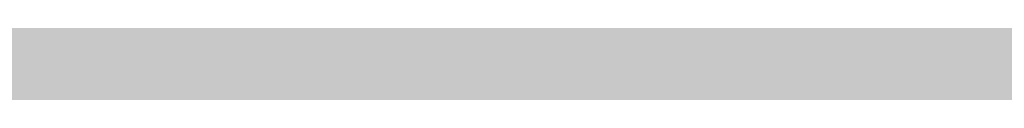
# Model space of a CAD drawing. Units: millimetres. Extents: x 0 to 2267, y 0 to 1823.
# Tile 173 of 256: x 1833.606 to 1838.83, y 1127.583 to 1127.888. Entities that reach past the tile are written whole.
import ezdxf

# ---------------------------------------------------------------- set-up
doc = ezdxf.new("R2010")
doc.units = ezdxf.units.MM
doc.header["$MEASUREMENT"] = 0
doc.layers.add('M-HATC', color=252, linetype='Continuous', lineweight=18)

msp = doc.modelspace()

# ---------------------------------------------------------------- hatches: boundary and pattern name
at = {"layer": 'M-HATC'}
h = msp.add_hatch(color=256, dxfattribs=at)
h.dxf.hatch_style = 1
h.paths.add_polyline_path([(2055.771, 1603.062), (1381.0868, 1603.062), (1381.0868, 1598.062), (2055.771, 1598.062)])
h.paths.add_polyline_path([(2055.771, 1598.062), (1381.0868, 1598.062), (1381.0868, 1593.062), (2055.771, 1593.062)])
h.paths.add_polyline_path([(2051.3074, 1536.7609), (1385.5504, 1536.7609), (1385.5504, 1526.7609), (1387.5504, 1526.7609), (1388.5366, 1525.0528), (1385.3319, 1521.2335), (1385.3319, 1521.2226), (2050.2542, 1522.7491), (2048.3212, 1525.0528), (2049.3074, 1526.7609), (2051.3074, 1526.7609)])
edge = h.paths.add_edge_path()
edge.add_arc((1847.5345, 1379.1492), 135, 222.603061, 222.890851, ccw=False)
edge.add_line((1748.1663, 1287.7656), (1683.0921, 1287.7656))
edge.add_arc((1583.7239, 1379.1492), 135, 317.109149, 317.396939, ccw=False)
edge.add_arc((1678.9686, 1290.6707), 5, 222.8909, 317.1091, ccw=False)
edge.add_arc((1774.2133, 1379.1492), 135, 222.603061, 222.890851, ccw=False)
edge.add_line((1674.8451, 1287.7656), (1609.7709, 1287.7656))
edge.add_arc((1510.4027, 1379.1492), 135, 317.109149, 317.396939, ccw=False)
edge.add_arc((1605.6474, 1290.6707), 5, 222.8909, 317.1091, ccw=False)
edge.add_arc((1700.8921, 1379.1492), 135, 222.603061, 222.890851, ccw=False)
edge.add_line((1601.5239, 1287.7656), (1536.4497, 1287.7656))
edge.add_arc((1437.0815, 1379.1492), 135, 317.109149, 317.396939, ccw=False)
edge.add_arc((1532.3262, 1290.6707), 5, 222.8909, 317.1091, ccw=False)
edge.add_arc((1627.5709, 1379.1492), 135, 222.603061, 222.890851, ccw=False)
edge.add_line((1528.2027, 1287.7656), (1505.9289, 1287.7656))
edge.add_spline(control_points=[(1505.9289, 1287.7656), (1504.2622, 1287.7656), (1504.2622, 1282.7656), (1505.9289, 1282.7656)], knot_values=[0, 0, 0, 0, 5, 5, 5, 5], degree=3, periodic=0)
edge.add_line((1505.9289, 1282.7656), (1930.9289, 1282.7656))
edge.add_spline(control_points=[(1930.9289, 1282.7656), (1932.5956, 1282.7656), (1932.5956, 1287.7656), (1930.9289, 1287.7656)], knot_values=[0, 0, 0, 0, 5, 5, 5, 5], degree=3, periodic=0)
edge.add_line((1930.9289, 1287.7656), (1903.0557, 1287.7656))
edge.add_arc((1803.6875, 1379.1492), 135, 317.109149, 317.396939, ccw=False)
edge.add_arc((1898.9322, 1290.6707), 5, 222.8909, 317.1091, ccw=False)
edge.add_arc((1994.1769, 1379.1492), 135, 222.603061, 222.890851, ccw=False)
edge.add_line((1894.8087, 1287.7656), (1829.7345, 1287.7656))
edge.add_arc((1730.3663, 1379.1492), 135, 317.109149, 317.396939, ccw=False)
edge.add_arc((1825.611, 1290.6707), 5, 222.8909, 317.1091, ccw=False)
edge.add_arc((1920.8557, 1379.1492), 135, 222.603061, 222.890851, ccw=False)
edge.add_line((1821.4875, 1287.7656), (1756.4133, 1287.7656))
edge.add_arc((1657.0451, 1379.1492), 135, 317.109149, 317.396939, ccw=False)
edge.add_arc((1752.2898, 1290.6707), 5, 222.8909, 317.1091, ccw=False)
edge = h.paths.add_edge_path()
edge.add_spline(control_points=[(1843.4289, 1227.2475), (1845.0956, 1227.2475), (1845.0956, 1232.2475), (1843.4289, 1232.2475)], knot_values=[0, 0, 0, 0, 5, 5, 5, 5], degree=3, periodic=0)
edge.add_line((1843.4289, 1232.2475), (1593.4289, 1232.2475))
edge.add_spline(control_points=[(1593.4289, 1232.2475), (1591.7622, 1232.2475), (1591.7622, 1227.2475), (1593.4289, 1227.2475)], knot_values=[0, 0, 0, 0, 5, 5, 5, 5], degree=3, periodic=0)
edge.add_line((1593.4289, 1227.2475), (1843.4289, 1227.2475))
h.paths.add_polyline_path([(1905.9289, 1127.4171), (1530.9289, 1127.4171, 0.414214), (1520.9289, 1117.4171), (1530.9289, 1117.4171), (1915.9289, 1117.4171, 0.414214)])
edge = h.paths.add_edge_path()
edge.add_arc((1397.0858, 1498.4078), 12.7299, 90.78215, 190.87871, ccw=False)
edge.add_line((1396.912, 1511.1365), (1428.0097, 1511.3488))
edge.add_line((1428.0097, 1511.3488), (1433.0097, 1511.3488))
edge.add_line((1433.0097, 1511.3488), (1434.439, 1511.3488))
edge.add_arc((1419.474, 1498.0804), 20, 41.561, 74.08211)
edge.add_line((1424.9592, 1517.3135), (1399.9351, 1517.2561))
edge.add_spline(control_points=[(1399.9307, 1517.2561), (1399.884, 1517.2131), (1399.8328, 1517.1689), (1399.7774, 1517.1236)], knot_values=[11.567499, 11.567499, 11.567499, 11.567499, 11.814249, 11.814249, 11.814249, 11.814249], degree=3, periodic=0)
edge.add_spline(control_points=[(1399.6328, 1517.0099), (1399.5831, 1516.9721), (1399.5307, 1516.9338), (1399.4759, 1516.8947)], knot_values=[11.167718, 11.167718, 11.167718, 11.167718, 11.365188, 11.365188, 11.365188, 11.365188], degree=3, periodic=0)
edge.add_spline(control_points=[(1399.3398, 1516.8001), (1399.1514, 1516.6719), (1398.9384, 1516.5377), (1398.704, 1516.3994)], knot_values=[10.376405, 10.376405, 10.376405, 10.376405, 11.00994, 11.00994, 11.00994, 11.00994], degree=3, periodic=0)
edge.add_spline(control_points=[(1398.6572, 1516.3719), (1398.5789, 1516.326), (1398.4983, 1516.2797), (1398.4155, 1516.2331)], knot_values=[10.125175, 10.125175, 10.125175, 10.125175, 10.334406, 10.334406, 10.334406, 10.334406], degree=3, periodic=0)
edge.add_spline(control_points=[(1398.2642, 1516.1487), (1398.196, 1516.1111), (1398.1263, 1516.0732), (1398.0555, 1516.0351)], knot_values=[9.832246, 9.832246, 9.832246, 9.832246, 9.999658, 9.999658, 9.999658, 9.999658], degree=3, periodic=0)
edge.add_spline(control_points=[(1397.9987, 1516.0048), (1397.7312, 1515.8621), (1397.446, 1515.7171), (1397.1466, 1515.5714)], knot_values=[9.161808, 9.161808, 9.161808, 9.161808, 9.787769, 9.787769, 9.787769, 9.787769], degree=3, periodic=0)
edge.add_spline(control_points=[(1397.1466, 1515.5714), (1396.8418, 1515.423), (1396.5222, 1515.274), (1396.1914, 1515.1262)], knot_values=[8.524455, 8.524455, 8.524455, 8.524455, 9.161808, 9.161808, 9.161808, 9.161808], degree=3, periodic=0)
edge.add_spline(control_points=[(1396.0777, 1515.0756), (1395.9854, 1515.0348), (1395.8922, 1514.994), (1395.7983, 1514.9534)], knot_values=[8.275193, 8.275193, 8.275193, 8.275193, 8.451726, 8.451726, 8.451726, 8.451726], degree=3, periodic=0)
edge.add_spline(control_points=[(1395.6018, 1514.8691), (1395.4997, 1514.8257), (1395.3968, 1514.7824), (1395.2932, 1514.7394)], knot_values=[7.962917, 7.962917, 7.962917, 7.962917, 8.152764, 8.152764, 8.152764, 8.152764], degree=3, periodic=0)
edge.add_spline(control_points=[(1395.2116, 1514.7057), (1394.8278, 1514.5475), (1394.4345, 1514.3929), (1394.0364, 1514.2442)], knot_values=[7.21254, 7.21254, 7.21254, 7.21254, 7.913148, 7.913148, 7.913148, 7.913148], degree=3, periodic=0)
edge.add_spline(control_points=[(1394.0364, 1514.2442), (1393.7076, 1514.1214), (1393.3754, 1514.0027), (1393.0427, 1513.8895)], knot_values=[6.633733, 6.633733, 6.633733, 6.633733, 7.21254, 7.21254, 7.21254, 7.21254], degree=3, periodic=0)
edge.add_spline(control_points=[(1392.8214, 1513.815), (1392.7198, 1513.7812), (1392.6181, 1513.7479), (1392.5166, 1513.7152)], knot_values=[6.328796, 6.328796, 6.328796, 6.328796, 6.505493, 6.505493, 6.505493, 6.505493], degree=3, periodic=0)
edge.add_spline(control_points=[(1392.5166, 1513.7152), (1392.3187, 1513.6515), (1392.1212, 1513.59), (1391.9244, 1513.531)], knot_values=[5.984605, 5.984605, 5.984605, 5.984605, 6.328796, 6.328796, 6.328796, 6.328796], degree=3, periodic=0)
edge.add_spline(control_points=[(1391.7915, 1513.4915), (1391.3122, 1513.3501), (1390.8384, 1513.2239), (1390.3784, 1513.1171)], knot_values=[5.066697, 5.066697, 5.066697, 5.066697, 5.907055, 5.907055, 5.907055, 5.907055], degree=3, periodic=0)
edge.add_spline(control_points=[(1390.3784, 1513.1171), (1390.1797, 1513.071), (1389.9836, 1513.0284), (1389.7907, 1512.9899)], knot_values=[4.70367, 4.70367, 4.70367, 4.70367, 5.066695, 5.066695, 5.066695, 5.066695], degree=3, periodic=0)
edge.add_spline(control_points=[(1389.422, 1512.9204), (1389.2459, 1512.8892), (1389.0729, 1512.8617), (1388.9036, 1512.8381)], knot_values=[4.130571, 4.130571, 4.130571, 4.130571, 4.469816, 4.469816, 4.469816, 4.469816], degree=3, periodic=0)
edge.add_spline(control_points=[(1388.9036, 1512.8381), (1388.591, 1512.7946), (1388.2911, 1512.7644), (1388.0071, 1512.7494)], knot_values=[3.504031, 3.504031, 3.504031, 3.504031, 4.130571, 4.130571, 4.130571, 4.130571], degree=3, periodic=0)
edge.add_spline(control_points=[(1387.9356, 1512.7459), (1387.8538, 1512.7423), (1387.7733, 1512.74), (1387.6944, 1512.739)], knot_values=[3.268866, 3.268866, 3.268866, 3.268866, 3.451164, 3.451164, 3.451164, 3.451164], degree=3, periodic=0)
edge.add_spline(control_points=[(1387.3351, 1512.7443), (1387.2076, 1512.7499), (1387.0847, 1512.7597), (1386.967, 1512.7739)], knot_values=[2.670686, 2.670686, 2.670686, 2.670686, 2.984, 2.984, 2.984, 2.984], degree=3, periodic=0)
edge.add_spline(control_points=[(1386.8327, 1512.7922), (1386.8209, 1512.7941), (1386.8092, 1512.7959), (1386.7975, 1512.7979)], knot_values=[2.516981, 2.516981, 2.516981, 2.516981, 2.549528, 2.549528, 2.549528, 2.549528], degree=3, periodic=0)
edge.add_spline(control_points=[(1386.4526, 1512.8735), (1386.4257, 1512.881), (1386.3993, 1512.889), (1386.3733, 1512.8972)], knot_values=[2.095869, 2.095869, 2.095869, 2.095869, 2.17941, 2.17941, 2.17941, 2.17941], degree=3, periodic=0)
edge.add_spline(control_points=[(1386.0691, 1513.0189), (1386.0634, 1513.0217), (1386.0577, 1513.0246), (1386.052, 1513.0275)], knot_values=[1.72453, 1.72453, 1.72453, 1.72453, 1.745933, 1.745933, 1.745933, 1.745933], degree=3, periodic=0)
edge.add_arc((1399.474, 1498.0804), 20, 131.82432, 180)
edge.add_arc((1630.3336, 1505.5484), 250.9708, 181.705176, 236.427975)
edge.add_arc((1605.3399, 1483.3044), 218.7822, 238.660829, 243.34961)
edge.add_arc((1647.0911, 1510.3592), 262.8986, 183.129836, 237.853442, ccw=False)
h.paths.add_polyline_path([(1406.5369, 1391.9644, 0.149382), (1491.5506, 1296.4418, -0.129517)], flags=17)
edge = h.paths.add_edge_path()
edge.add_arc((2037.3838, 1498.0804), 20, 0, 48.26587)
edge.add_spline(control_points=[(2050.6973, 1513.0052), (2050.6512, 1512.9847), (2050.6034, 1512.9655), (2050.5539, 1512.9477)], knot_values=[1.835652, 1.835652, 1.835652, 1.835652, 2.000781, 2.000781, 2.000781, 2.000781], degree=3, periodic=0)
edge.add_spline(control_points=[(2050.4616, 1512.9166), (2050.479, 1512.9221), (2050.4963, 1512.9277), (2050.5133, 1512.9335)], knot_values=[2.045477, 2.045477, 2.045477, 2.045477, 2.101389, 2.101389, 2.101389, 2.101389], degree=3, periodic=0)
edge.add_spline(control_points=[(2050.129, 1512.8342), (2050.1984, 1512.8473), (2050.2657, 1512.8623), (2050.3308, 1512.8792)], knot_values=[2.237629, 2.237629, 2.237629, 2.237629, 2.435841, 2.435841, 2.435841, 2.435841], degree=3, periodic=0)
edge.add_spline(control_points=[(2050.0946, 1512.8278), (2050.1061, 1512.8299), (2050.1176, 1512.832), (2050.129, 1512.8342)], knot_values=[2.435841, 2.435841, 2.435841, 2.435841, 2.468321, 2.468321, 2.468321, 2.468321], degree=3, periodic=0)
edge.add_spline(control_points=[(2049.7843, 1512.7851), (2049.8552, 1512.7922), (2049.9243, 1512.8008), (2049.9917, 1512.8109)], knot_values=[2.563852, 2.563852, 2.563852, 2.563852, 2.748541, 2.748541, 2.748541, 2.748541], degree=3, periodic=0)
edge.add_spline(control_points=[(2049.4052, 1512.7617), (2049.5364, 1512.7653), (2049.6629, 1512.773), (2049.7843, 1512.7851)], knot_values=[2.748541, 2.748541, 2.748541, 2.748541, 3.064882, 3.064882, 3.064882, 3.064882], degree=3, periodic=0)
edge.add_spline(control_points=[(2049.1698, 1512.7597), (2049.2336, 1512.7591), (2049.2965, 1512.7594), (2049.3584, 1512.7606)], knot_values=[3.102309, 3.102309, 3.102309, 3.102309, 3.2503, 3.2503, 3.2503, 3.2503], degree=3, periodic=0)
edge.add_spline(control_points=[(2048.8573, 1512.7691), (2048.9638, 1512.7638), (2049.068, 1512.7606), (2049.1698, 1512.7597)], knot_values=[3.2503, 3.2503, 3.2503, 3.2503, 3.486069, 3.486069, 3.486069, 3.486069], degree=3, periodic=0)
edge.add_spline(control_points=[(2048.6924, 1512.7789), (2048.3729, 1512.8009), (2048.0345, 1512.8411), (2047.6817, 1512.897)], knot_values=[3.606429, 3.606429, 3.606429, 3.606429, 4.2989, 4.2989, 4.2989, 4.2989], degree=3, periodic=0)
edge.add_spline(control_points=[(2047.6817, 1512.897), (2047.5458, 1512.9185), (2047.4077, 1512.9424), (2047.2678, 1512.9685)], knot_values=[4.2989, 4.2989, 4.2989, 4.2989, 4.565769, 4.565769, 4.565769, 4.565769], degree=3, periodic=0)
edge.add_spline(control_points=[(2047.2678, 1512.9685), (2047.1449, 1512.9914), (2047.0207, 1513.016), (2046.8951, 1513.0422)], knot_values=[4.565769, 4.565769, 4.565769, 4.565769, 4.799971, 4.799971, 4.799971, 4.799971], degree=3, periodic=0)
edge.add_spline(control_points=[(2046.8951, 1513.0422), (2046.5286, 1513.1188), (2046.1513, 1513.209), (2045.7676, 1513.3107)], knot_values=[4.799971, 4.799971, 4.799971, 4.799971, 5.483718, 5.483718, 5.483718, 5.483718], degree=3, periodic=0)
edge.add_spline(control_points=[(2045.7676, 1513.3107), (2045.3724, 1513.4154), (2044.9704, 1513.5322), (2044.5662, 1513.6588)], knot_values=[5.483718, 5.483718, 5.483718, 5.483718, 6.187866, 6.187866, 6.187866, 6.187866], degree=3, periodic=0)
edge.add_spline(control_points=[(2044.5662, 1513.6588), (2044.4149, 1513.7061), (2044.2633, 1513.7549), (2044.1116, 1513.8048)], knot_values=[6.187866, 6.187866, 6.187866, 6.187866, 6.451551, 6.451551, 6.451551, 6.451551], degree=3, periodic=0)
edge.add_spline(control_points=[(2044.1116, 1513.8048), (2043.9967, 1513.8427), (2043.8817, 1513.8813), (2043.7668, 1513.9205)], knot_values=[6.451551, 6.451551, 6.451551, 6.451551, 6.651434, 6.651434, 6.651434, 6.651434], degree=3, periodic=0)
edge.add_spline(control_points=[(2043.7668, 1513.9205), (2043.3716, 1514.0554), (2042.9774, 1514.1979), (2042.5886, 1514.3458)], knot_values=[6.651434, 6.651434, 6.651434, 6.651434, 7.338879, 7.338879, 7.338879, 7.338879], degree=3, periodic=0)
edge.add_spline(control_points=[(2042.5886, 1514.3458), (2042.1643, 1514.5071), (2041.7465, 1514.6749), (2041.3409, 1514.846)], knot_values=[7.338879, 7.338879, 7.338879, 7.338879, 8.089209, 8.089209, 8.089209, 8.089209], degree=3, periodic=0)
edge.add_spline(control_points=[(2041.3409, 1514.846), (2041.1028, 1514.9465), (2040.869, 1515.0481), (2040.6405, 1515.1502)], knot_values=[8.089209, 8.089209, 8.089209, 8.089209, 8.529587, 8.529587, 8.529587, 8.529587], degree=3, periodic=0)
edge.add_spline(control_points=[(2040.51, 1515.2089), (2040.0824, 1515.4022), (2039.6747, 1515.5971), (2039.295, 1515.7894)], knot_values=[8.613818, 8.613818, 8.613818, 8.613818, 9.44571, 9.44571, 9.44571, 9.44571], degree=3, periodic=0)
edge.add_spline(control_points=[(2039.295, 1515.7894), (2039.0618, 1515.9075), (2038.8391, 1516.0246), (2038.6288, 1516.1398)], knot_values=[9.44571, 9.44571, 9.44571, 9.44571, 9.956404, 9.956404, 9.956404, 9.956404], degree=3, periodic=0)
edge.add_spline(control_points=[(2038.6288, 1516.1398), (2038.5187, 1516.2001), (2038.4121, 1516.2598), (2038.309, 1516.3189)], knot_values=[9.956404, 9.956404, 9.956404, 9.956404, 10.223542, 10.223542, 10.223542, 10.223542], degree=3, periodic=0)
edge.add_spline(control_points=[(2038.309, 1516.3189), (2038.2138, 1516.3735), (2038.1216, 1516.4276), (2038.0328, 1516.481)], knot_values=[10.223542, 10.223542, 10.223542, 10.223542, 10.47051, 10.47051, 10.47051, 10.47051], degree=3, periodic=0)
edge.add_spline(control_points=[(2038.0328, 1516.481), (2037.7855, 1516.6296), (2037.5639, 1516.773), (2037.3722, 1516.909)], knot_values=[10.47051, 10.47051, 10.47051, 10.47051, 11.15767, 11.15767, 11.15767, 11.15767], degree=3, periodic=0)
edge.add_spline(control_points=[(2037.3722, 1516.909), (2037.2789, 1516.9752), (2037.1927, 1517.0396), (2037.1142, 1517.102)], knot_values=[11.15767, 11.15767, 11.15767, 11.15767, 11.49227, 11.49227, 11.49227, 11.49227], degree=3, periodic=0)
edge.add_spline(control_points=[(2036.8564, 1517.3259), (2036.9148, 1517.2692), (2036.9814, 1517.2103), (2037.0557, 1517.1492)], knot_values=[11.577341, 11.577341, 11.577341, 11.577341, 11.91035, 11.91035, 11.91035, 11.91035], degree=3, periodic=0)
edge.add_spline(control_points=[(2036.8074, 1517.3748), (2036.823, 1517.3587), (2036.8393, 1517.3424), (2036.8564, 1517.3259)], knot_values=[11.91035, 11.91035, 11.91035, 11.91035, 12.007402, 12.007402, 12.007402, 12.007402], degree=3, periodic=0)
edge.add_spline(control_points=[(2036.7017, 1517.494), (2036.7104, 1517.483), (2036.7196, 1517.4719), (2036.7291, 1517.4606)], knot_values=[12.184155, 12.184155, 12.184155, 12.184155, 12.255409, 12.255409, 12.255409, 12.255409], degree=3, periodic=0)
edge.add_spline(control_points=[(2036.6159, 1517.6205), (2036.62, 1517.613), (2036.6243, 1517.6055), (2036.6289, 1517.5979)], knot_values=[12.487913, 12.487913, 12.487913, 12.487913, 12.541035, 12.541035, 12.541035, 12.541035], degree=3, periodic=0)
edge.add_spline(control_points=[(2036.5635, 1517.786), (2036.5637, 1517.7794), (2036.5642, 1517.7726), (2036.565, 1517.7658)], knot_values=[12.911761, 12.911761, 12.911761, 12.911761, 12.968286, 12.968286, 12.968286, 12.968286], degree=3, periodic=0)
edge.add_spline(control_points=[(2036.6166, 1517.9304), (2036.6125, 1517.9259), (2036.6086, 1517.9212), (2036.6049, 1517.9165)], knot_values=[13.382527, 13.382527, 13.382527, 13.382527, 13.433791, 13.433791, 13.433791, 13.433791], degree=3, periodic=0)
edge.add_spline(control_points=[(2036.749, 1518.017), (2036.7361, 1518.0116), (2036.7239, 1518.006), (2036.7124, 1518.0002)], knot_values=[13.726299, 13.726299, 13.726299, 13.726299, 13.809928, 13.809928, 13.809928, 13.809928], degree=3, periodic=0)
edge.add_spline(control_points=[(2036.8604, 1518.0528), (2036.8386, 1518.0474), (2036.8181, 1518.0416), (2036.7988, 1518.0353)], knot_values=[13.910887, 13.910887, 13.910887, 13.910887, 14.02153, 14.02153, 14.02153, 14.02153], degree=3, periodic=0)
edge.add_line((2036.9639, 1518.0804), (2032.3838, 1518.0804))
edge.add_line((2032.3838, 1518.0804), (2027.3838, 1518.0804))
edge.add_line((2027.3838, 1518.0804), (2022.3838, 1518.0804))
edge.add_line((2022.3838, 1518.0804), (2017.3838, 1518.0804))
edge.add_arc((2017.3838, 1498.0804), 20, 90, 138.439)
edge.add_line((2002.4188, 1511.3488), (2003.8481, 1511.3488))
edge.add_line((2003.8481, 1511.3488), (2008.8481, 1511.3488))
edge.add_line((2008.8481, 1511.3488), (2039.772, 1511.1377))
edge.add_arc((2039.772, 1498.4078), 12.7299, -10.87871, 90, ccw=False)
edge.add_arc((1789.7668, 1510.3592), 262.8986, 302.146558, 356.870164, ccw=False)
edge.add_arc((1831.5179, 1483.3044), 218.7822, 296.65039, 301.339171)
edge.add_arc((1806.5242, 1505.5484), 250.9708, 303.572025, 358.294824)
h.paths.add_polyline_path([(2030.321, 1391.9644, -0.129517), (1945.3072, 1296.4418, 0.149382)], flags=17)
edge = h.paths.add_edge_path()
edge.add_spline(control_points=[(2037.2464, 1518.0821), (2037.2898, 1518.081), (2037.3355, 1518.0804), (2037.3838, 1518.0804)], knot_values=[0.000012, 0.000012, 0.000012, 0.000012, 0.144754, 0.144754, 0.144754, 0.144754], degree=3, periodic=0)
edge.add_line((2037.3357, 1518.0804), (2037.0096, 1518.0804))
edge.add_spline(control_points=[(2037.0096, 1518.0804), (2036.9822, 1518.0768), (2036.956, 1518.0727), (2036.9312, 1518.0681)], knot_values=[14.13465, 14.13465, 14.13465, 14.13465, 14.247197, 14.247197, 14.247197, 14.247197], degree=3, periodic=0)
edge.add_spline(control_points=[(2036.9312, 1518.0681), (2036.9276, 1518.0674), (2036.9241, 1518.0667), (2036.9205, 1518.0661)], knot_values=[14.118315, 14.118315, 14.118315, 14.118315, 14.13465, 14.13465, 14.13465, 14.13465], degree=3, periodic=0)
edge.add_spline(control_points=[(2036.9205, 1518.0661), (2036.9118, 1518.0644), (2036.9032, 1518.0626), (2036.8948, 1518.0608)], knot_values=[14.078086, 14.078086, 14.078086, 14.078086, 14.118315, 14.118315, 14.118315, 14.118315], degree=3, periodic=0)
edge.add_spline(control_points=[(2036.8948, 1518.0608), (2036.883, 1518.0583), (2036.8716, 1518.0556), (2036.8604, 1518.0528)], knot_values=[14.02153, 14.02153, 14.02153, 14.02153, 14.078086, 14.078086, 14.078086, 14.078086], degree=3, periodic=0)
edge.add_spline(control_points=[(2036.8604, 1518.0528), (2036.8386, 1518.0474), (2036.8181, 1518.0416), (2036.7988, 1518.0353)], knot_values=[13.910887, 13.910887, 13.910887, 13.910887, 14.02153, 14.02153, 14.02153, 14.02153], degree=3, periodic=0)
edge.add_spline(control_points=[(2036.7988, 1518.0353), (2036.7981, 1518.035), (2036.7974, 1518.0348), (2036.7967, 1518.0346)], knot_values=[13.906906, 13.906906, 13.906906, 13.906906, 13.910887, 13.910887, 13.910887, 13.910887], degree=3, periodic=0)
edge.add_spline(control_points=[(2036.7967, 1518.0346), (2036.7882, 1518.0318), (2036.7799, 1518.0289), (2036.7719, 1518.0259)], knot_values=[13.857826, 13.857826, 13.857826, 13.857826, 13.906906, 13.906906, 13.906906, 13.906906], degree=3, periodic=0)
edge.add_spline(control_points=[(2036.7719, 1518.0259), (2036.764, 1518.023), (2036.7564, 1518.02), (2036.749, 1518.017)], knot_values=[13.809928, 13.809928, 13.809928, 13.809928, 13.857826, 13.857826, 13.857826, 13.857826], degree=3, periodic=0)
edge.add_spline(control_points=[(2036.749, 1518.017), (2036.7361, 1518.0116), (2036.7239, 1518.006), (2036.7124, 1518.0002)], knot_values=[13.726299, 13.726299, 13.726299, 13.726299, 13.809928, 13.809928, 13.809928, 13.809928], degree=3, periodic=0)
edge.add_spline(control_points=[(2036.7124, 1518.0002), (2036.7121, 1518), (2036.7118, 1517.9999), (2036.7115, 1517.9997)], knot_values=[13.723993, 13.723993, 13.723993, 13.723993, 13.726299, 13.726299, 13.726299, 13.726299], degree=3, periodic=0)
edge.add_spline(control_points=[(2036.7115, 1517.9997), (2036.7063, 1517.9971), (2036.7013, 1517.9944), (2036.6965, 1517.9917)], knot_values=[13.686536, 13.686536, 13.686536, 13.686536, 13.723993, 13.723993, 13.723993, 13.723993], degree=3, periodic=0)
edge.add_spline(control_points=[(2036.6965, 1517.9917), (2036.6919, 1517.9891), (2036.6874, 1517.9865), (2036.6831, 1517.9839)], knot_values=[13.651251, 13.651251, 13.651251, 13.651251, 13.686536, 13.686536, 13.686536, 13.686536], degree=3, periodic=0)
edge.add_spline(control_points=[(2036.6831, 1517.9839), (2036.6764, 1517.9798), (2036.67, 1517.9757), (2036.6639, 1517.9714)], knot_values=[13.596804, 13.596804, 13.596804, 13.596804, 13.651251, 13.651251, 13.651251, 13.651251], degree=3, periodic=0)
edge.add_spline(control_points=[(2036.6639, 1517.9714), (2036.6636, 1517.9712), (2036.6633, 1517.9709), (2036.6629, 1517.9707)], knot_values=[13.593956, 13.593956, 13.593956, 13.593956, 13.596804, 13.596804, 13.596804, 13.596804], degree=3, periodic=0)
edge.add_spline(control_points=[(2036.6629, 1517.9707), (2036.6603, 1517.9689), (2036.6577, 1517.967), (2036.6552, 1517.9651)], knot_values=[13.570322, 13.570322, 13.570322, 13.570322, 13.593956, 13.593956, 13.593956, 13.593956], degree=3, periodic=0)
edge.add_spline(control_points=[(2036.6552, 1517.9651), (2036.6525, 1517.9631), (2036.6499, 1517.9611), (2036.6474, 1517.9591)], knot_values=[13.545477, 13.545477, 13.545477, 13.545477, 13.570322, 13.570322, 13.570322, 13.570322], degree=3, periodic=0)
edge.add_spline(control_points=[(2036.6474, 1517.9591), (2036.6472, 1517.9589), (2036.6471, 1517.9588), (2036.6469, 1517.9587)], knot_values=[13.543931, 13.543931, 13.543931, 13.543931, 13.545477, 13.545477, 13.545477, 13.545477], degree=3, periodic=0)
edge.add_spline(control_points=[(2036.6469, 1517.9587), (2036.6412, 1517.9541), (2036.6358, 1517.9494), (2036.6307, 1517.9447)], knot_values=[13.488237, 13.488237, 13.488237, 13.488237, 13.543931, 13.543931, 13.543931, 13.543931], degree=3, periodic=0)
edge.add_spline(control_points=[(2036.6307, 1517.9447), (2036.6282, 1517.9423), (2036.6257, 1517.9399), (2036.6233, 1517.9374)], knot_values=[13.460307, 13.460307, 13.460307, 13.460307, 13.488237, 13.488237, 13.488237, 13.488237], degree=3, periodic=0)
edge.add_spline(control_points=[(2036.6233, 1517.9374), (2036.6215, 1517.9356), (2036.6198, 1517.9338), (2036.6181, 1517.932)], knot_values=[13.439712, 13.439712, 13.439712, 13.439712, 13.460307, 13.460307, 13.460307, 13.460307], degree=3, periodic=0)
edge.add_spline(control_points=[(2036.6181, 1517.932), (2036.6176, 1517.9315), (2036.6171, 1517.9309), (2036.6166, 1517.9304)], knot_values=[13.433791, 13.433791, 13.433791, 13.433791, 13.439712, 13.439712, 13.439712, 13.439712], degree=3, periodic=0)
edge.add_spline(control_points=[(2036.6166, 1517.9304), (2036.6125, 1517.9259), (2036.6086, 1517.9212), (2036.6049, 1517.9165)], knot_values=[13.382527, 13.382527, 13.382527, 13.382527, 13.433791, 13.433791, 13.433791, 13.433791], degree=3, periodic=0)
edge.add_spline(control_points=[(2036.6049, 1517.9165), (2036.6026, 1517.9135), (2036.6004, 1517.9104), (2036.5982, 1517.9074)], knot_values=[13.350017, 13.350017, 13.350017, 13.350017, 13.382527, 13.382527, 13.382527, 13.382527], degree=3, periodic=0)
edge.add_spline(control_points=[(2036.5982, 1517.9074), (2036.5972, 1517.9059), (2036.5962, 1517.9043), (2036.5952, 1517.9028)], knot_values=[13.333922, 13.333922, 13.333922, 13.333922, 13.350017, 13.350017, 13.350017, 13.350017], degree=3, periodic=0)
edge.add_spline(control_points=[(2036.5952, 1517.9028), (2036.5945, 1517.9018), (2036.5939, 1517.9009), (2036.5933, 1517.8999)], knot_values=[13.323828, 13.323828, 13.323828, 13.323828, 13.333922, 13.333922, 13.333922, 13.333922], degree=3, periodic=0)
edge.add_spline(control_points=[(2036.5933, 1517.8999), (2036.5905, 1517.8955), (2036.5879, 1517.8909), (2036.5855, 1517.8864)], knot_values=[13.277545, 13.277545, 13.277545, 13.277545, 13.323828, 13.323828, 13.323828, 13.323828], degree=3, periodic=0)
edge.add_spline(control_points=[(2036.5855, 1517.8864), (2036.5836, 1517.8827), (2036.5817, 1517.8789), (2036.5801, 1517.8751)], knot_values=[13.240119, 13.240119, 13.240119, 13.240119, 13.277545, 13.277545, 13.277545, 13.277545], degree=3, periodic=0)
edge.add_spline(control_points=[(2036.5801, 1517.8751), (2036.5795, 1517.8739), (2036.579, 1517.8727), (2036.5785, 1517.8715)], knot_values=[13.228211, 13.228211, 13.228211, 13.228211, 13.240119, 13.240119, 13.240119, 13.240119], degree=3, periodic=0)
edge.add_spline(control_points=[(2036.5785, 1517.8715), (2036.578, 1517.8702), (2036.5774, 1517.869), (2036.5769, 1517.8677)], knot_values=[13.215717, 13.215717, 13.215717, 13.215717, 13.228211, 13.228211, 13.228211, 13.228211], degree=3, periodic=0)
edge.add_spline(control_points=[(2036.5769, 1517.8677), (2036.5755, 1517.864), (2036.5741, 1517.8603), (2036.5729, 1517.8565)], knot_values=[13.179847, 13.179847, 13.179847, 13.179847, 13.215717, 13.215717, 13.215717, 13.215717], degree=3, periodic=0)
edge.add_spline(control_points=[(2036.5729, 1517.8565), (2036.5713, 1517.8515), (2036.5699, 1517.8464), (2036.5687, 1517.8413)], knot_values=[13.132017, 13.132017, 13.132017, 13.132017, 13.179847, 13.179847, 13.179847, 13.179847], degree=3, periodic=0)
edge.add_spline(control_points=[(2036.5687, 1517.8413), (2036.5684, 1517.8402), (2036.5682, 1517.8392), (2036.568, 1517.8382)], knot_values=[13.122482, 13.122482, 13.122482, 13.122482, 13.132017, 13.132017, 13.132017, 13.132017], degree=3, periodic=0)
edge.add_spline(control_points=[(2036.568, 1517.8382), (2036.5676, 1517.8363), (2036.5672, 1517.8345), (2036.5669, 1517.8327)], knot_values=[13.105592, 13.105592, 13.105592, 13.105592, 13.122482, 13.122482, 13.122482, 13.122482], degree=3, periodic=0)
edge.add_spline(control_points=[(2036.5669, 1517.8327), (2036.5662, 1517.8292), (2036.5657, 1517.8257), (2036.5652, 1517.8222)], knot_values=[13.074063, 13.074063, 13.074063, 13.074063, 13.105592, 13.105592, 13.105592, 13.105592], degree=3, periodic=0)
edge.add_spline(control_points=[(2036.5652, 1517.8222), (2036.5652, 1517.8222), (2036.5652, 1517.8222), (2036.5652, 1517.8222)], knot_values=[13.074043, 13.074043, 13.074043, 13.074043, 13.074063, 13.074063, 13.074063, 13.074063], degree=3, periodic=0)
edge.add_spline(control_points=[(2036.5652, 1517.8222), (2036.5644, 1517.8164), (2036.5639, 1517.8106), (2036.5636, 1517.8046)], knot_values=[13.021884, 13.021884, 13.021884, 13.021884, 13.074043, 13.074043, 13.074043, 13.074043], degree=3, periodic=0)
edge.add_spline(control_points=[(2036.5636, 1517.8046), (2036.5636, 1517.804), (2036.5636, 1517.8034), (2036.5635, 1517.8028)], knot_values=[13.01674, 13.01674, 13.01674, 13.01674, 13.021884, 13.021884, 13.021884, 13.021884], degree=3, periodic=0)
edge.add_spline(control_points=[(2036.5635, 1517.8028), (2036.5634, 1517.8005), (2036.5634, 1517.7982), (2036.5634, 1517.7958)], knot_values=[12.996438, 12.996438, 12.996438, 12.996438, 13.01674, 13.01674, 13.01674, 13.01674], degree=3, periodic=0)
edge.add_spline(control_points=[(2036.5634, 1517.7958), (2036.5633, 1517.7926), (2036.5634, 1517.7893), (2036.5635, 1517.786)], knot_values=[12.968286, 12.968286, 12.968286, 12.968286, 12.996438, 12.996438, 12.996438, 12.996438], degree=3, periodic=0)
edge.add_spline(control_points=[(2036.5635, 1517.786), (2036.5637, 1517.7794), (2036.5642, 1517.7726), (2036.565, 1517.7658)], knot_values=[12.911761, 12.911761, 12.911761, 12.911761, 12.968286, 12.968286, 12.968286, 12.968286], degree=3, periodic=0)
edge.add_spline(control_points=[(2036.565, 1517.7658), (2036.565, 1517.7657), (2036.565, 1517.7656), (2036.565, 1517.7656)], knot_values=[12.911017, 12.911017, 12.911017, 12.911017, 12.911761, 12.911761, 12.911761, 12.911761], degree=3, periodic=0)
edge.add_spline(control_points=[(2036.565, 1517.7656), (2036.5654, 1517.7625), (2036.5658, 1517.7593), (2036.5663, 1517.7562)], knot_values=[12.88528, 12.88528, 12.88528, 12.88528, 12.911017, 12.911017, 12.911017, 12.911017], degree=3, periodic=0)
edge.add_spline(control_points=[(2036.5663, 1517.7562), (2036.5667, 1517.7534), (2036.5672, 1517.7506), (2036.5677, 1517.7478)], knot_values=[12.862519, 12.862519, 12.862519, 12.862519, 12.88528, 12.88528, 12.88528, 12.88528], degree=3, periodic=0)
edge.add_spline(control_points=[(2036.5677, 1517.7478), (2036.5678, 1517.7474), (2036.5679, 1517.7469), (2036.568, 1517.7465)], knot_values=[12.858885, 12.858885, 12.858885, 12.858885, 12.862519, 12.862519, 12.862519, 12.862519], degree=3, periodic=0)
edge.add_spline(control_points=[(2036.568, 1517.7465), (2036.5692, 1517.7399), (2036.5707, 1517.7332), (2036.5724, 1517.7264)], knot_values=[12.8053, 12.8053, 12.8053, 12.8053, 12.858885, 12.858885, 12.858885, 12.858885], degree=3, periodic=0)
edge.add_spline(control_points=[(2036.5724, 1517.7264), (2036.5734, 1517.7226), (2036.5745, 1517.7187), (2036.5756, 1517.7149)], knot_values=[12.775176, 12.775176, 12.775176, 12.775176, 12.8053, 12.8053, 12.8053, 12.8053], degree=3, periodic=0)
edge.add_spline(control_points=[(2036.5756, 1517.7149), (2036.5763, 1517.7125), (2036.577, 1517.7102), (2036.5778, 1517.7078)], knot_values=[12.756759, 12.756759, 12.756759, 12.756759, 12.775176, 12.775176, 12.775176, 12.775176], degree=3, periodic=0)
edge.add_spline(control_points=[(2036.5778, 1517.7078), (2036.5781, 1517.7067), (2036.5784, 1517.7057), (2036.5787, 1517.7047)], knot_values=[12.748742, 12.748742, 12.748742, 12.748742, 12.756759, 12.756759, 12.756759, 12.756759], degree=3, periodic=0)
edge.add_spline(control_points=[(2036.5787, 1517.7047), (2036.5808, 1517.6983), (2036.5831, 1517.6919), (2036.5856, 1517.6854)], knot_values=[12.69959, 12.69959, 12.69959, 12.69959, 12.748742, 12.748742, 12.748742, 12.748742], degree=3, periodic=0)
edge.add_spline(control_points=[(2036.5856, 1517.6854), (2036.5876, 1517.68), (2036.5898, 1517.6746), (2036.5921, 1517.6692)], knot_values=[12.659038, 12.659038, 12.659038, 12.659038, 12.69959, 12.69959, 12.69959, 12.69959], degree=3, periodic=0)
edge.add_spline(control_points=[(2036.5921, 1517.6692), (2036.594, 1517.6648), (2036.5959, 1517.6605), (2036.5979, 1517.6561)], knot_values=[12.626806, 12.626806, 12.626806, 12.626806, 12.659038, 12.659038, 12.659038, 12.659038], degree=3, periodic=0)
edge.add_spline(control_points=[(2036.5979, 1517.6561), (2036.5984, 1517.6551), (2036.5989, 1517.6541), (2036.5993, 1517.6531)], knot_values=[12.619394, 12.619394, 12.619394, 12.619394, 12.626806, 12.626806, 12.626806, 12.626806], degree=3, periodic=0)
edge.add_spline(control_points=[(2036.5993, 1517.6531), (2036.6043, 1517.6424), (2036.6099, 1517.6315), (2036.6159, 1517.6205)], knot_values=[12.541039, 12.541039, 12.541039, 12.541039, 12.619394, 12.619394, 12.619394, 12.619394], degree=3, periodic=0)
edge.add_spline(control_points=[(2036.6159, 1517.6205), (2036.6159, 1517.6205), (2036.6159, 1517.6205), (2036.6159, 1517.6205)], knot_values=[12.541035, 12.541035, 12.541035, 12.541035, 12.541039, 12.541039, 12.541039, 12.541039], degree=3, periodic=0)
edge.add_spline(control_points=[(2036.6159, 1517.6205), (2036.62, 1517.613), (2036.6243, 1517.6055), (2036.6289, 1517.5979)], knot_values=[12.487913, 12.487913, 12.487913, 12.487913, 12.541035, 12.541035, 12.541035, 12.541035], degree=3, periodic=0)
edge.add_spline(control_points=[(2036.6289, 1517.5979), (2036.6326, 1517.5916), (2036.6365, 1517.5853), (2036.6406, 1517.5789)], knot_values=[12.443982, 12.443982, 12.443982, 12.443982, 12.487913, 12.487913, 12.487913, 12.487913], degree=3, periodic=0)
edge.add_spline(control_points=[(2036.6406, 1517.5789), (2036.6414, 1517.5776), (2036.6423, 1517.5763), (2036.6431, 1517.5749)], knot_values=[12.434996, 12.434996, 12.434996, 12.434996, 12.443982, 12.443982, 12.443982, 12.443982], degree=3, periodic=0)
edge.add_spline(control_points=[(2036.6431, 1517.5749), (2036.6531, 1517.5596), (2036.6639, 1517.5439), (2036.6756, 1517.528)], knot_values=[12.329647, 12.329647, 12.329647, 12.329647, 12.434996, 12.434996, 12.434996, 12.434996], degree=3, periodic=0)
edge.add_spline(control_points=[(2036.6756, 1517.528), (2036.6839, 1517.5168), (2036.6925, 1517.5055), (2036.7017, 1517.494)], knot_values=[12.255409, 12.255409, 12.255409, 12.255409, 12.329647, 12.329647, 12.329647, 12.329647], degree=3, periodic=0)
edge.add_spline(control_points=[(2036.7017, 1517.494), (2036.7104, 1517.483), (2036.7196, 1517.4719), (2036.7291, 1517.4606)], knot_values=[12.184155, 12.184155, 12.184155, 12.184155, 12.255409, 12.255409, 12.255409, 12.255409], degree=3, periodic=0)
edge.add_spline(control_points=[(2036.7291, 1517.4606), (2036.7436, 1517.4435), (2036.759, 1517.4262), (2036.7753, 1517.4085)], knot_values=[12.075961, 12.075961, 12.075961, 12.075961, 12.184155, 12.184155, 12.184155, 12.184155], degree=3, periodic=0)
edge.add_spline(control_points=[(2036.7753, 1517.4085), (2036.7763, 1517.4075), (2036.7773, 1517.4064), (2036.7783, 1517.4054)], knot_values=[12.069502, 12.069502, 12.069502, 12.069502, 12.075961, 12.075961, 12.075961, 12.075961], degree=3, periodic=0)
edge.add_spline(control_points=[(2036.7783, 1517.4054), (2036.7877, 1517.3953), (2036.7974, 1517.385), (2036.8074, 1517.3748)], knot_values=[12.007402, 12.007402, 12.007402, 12.007402, 12.069502, 12.069502, 12.069502, 12.069502], degree=3, periodic=0)
edge.add_spline(control_points=[(2036.8074, 1517.3748), (2036.823, 1517.3587), (2036.8393, 1517.3424), (2036.8564, 1517.3259)], knot_values=[11.91035, 11.91035, 11.91035, 11.91035, 12.007402, 12.007402, 12.007402, 12.007402], degree=3, periodic=0)
edge.add_spline(control_points=[(2036.8564, 1517.3259), (2036.9148, 1517.2692), (2036.9814, 1517.2103), (2037.0557, 1517.1492)], knot_values=[11.577341, 11.577341, 11.577341, 11.577341, 11.91035, 11.91035, 11.91035, 11.91035], degree=3, periodic=0)
edge.add_spline(control_points=[(2037.0557, 1517.1492), (2037.0747, 1517.1336), (2037.0942, 1517.1179), (2037.1142, 1517.102)], knot_values=[11.49227, 11.49227, 11.49227, 11.49227, 11.577341, 11.577341, 11.577341, 11.577341], degree=3, periodic=0)
edge.add_spline(control_points=[(2037.1142, 1517.102), (2037.1927, 1517.0396), (2037.2789, 1516.9752), (2037.3722, 1516.909)], knot_values=[11.15767, 11.15767, 11.15767, 11.15767, 11.49227, 11.49227, 11.49227, 11.49227], degree=3, periodic=0)
edge.add_spline(control_points=[(2037.3722, 1516.909), (2037.5639, 1516.773), (2037.7855, 1516.6296), (2038.0328, 1516.481)], knot_values=[10.47051, 10.47051, 10.47051, 10.47051, 11.15767, 11.15767, 11.15767, 11.15767], degree=3, periodic=0)
edge.add_spline(control_points=[(2038.0328, 1516.481), (2038.1216, 1516.4276), (2038.2138, 1516.3735), (2038.309, 1516.3189)], knot_values=[10.223542, 10.223542, 10.223542, 10.223542, 10.47051, 10.47051, 10.47051, 10.47051], degree=3, periodic=0)
edge.add_spline(control_points=[(2038.309, 1516.3189), (2038.4121, 1516.2598), (2038.5187, 1516.2001), (2038.6288, 1516.1398)], knot_values=[9.956404, 9.956404, 9.956404, 9.956404, 10.223542, 10.223542, 10.223542, 10.223542], degree=3, periodic=0)
edge.add_spline(control_points=[(2038.6288, 1516.1398), (2038.8391, 1516.0246), (2039.0618, 1515.9075), (2039.295, 1515.7894)], knot_values=[9.44571, 9.44571, 9.44571, 9.44571, 9.956404, 9.956404, 9.956404, 9.956404], degree=3, periodic=0)
edge.add_spline(control_points=[(2039.295, 1515.7894), (2039.6747, 1515.5971), (2040.0824, 1515.4022), (2040.51, 1515.2089)], knot_values=[8.613818, 8.613818, 8.613818, 8.613818, 9.44571, 9.44571, 9.44571, 9.44571], degree=3, periodic=0)
edge.add_spline(control_points=[(2040.51, 1515.2089), (2040.5533, 1515.1893), (2040.5968, 1515.1697), (2040.6405, 1515.1502)], knot_values=[8.529587, 8.529587, 8.529587, 8.529587, 8.613818, 8.613818, 8.613818, 8.613818], degree=3, periodic=0)
edge.add_spline(control_points=[(2040.6405, 1515.1502), (2040.869, 1515.0481), (2041.1028, 1514.9465), (2041.3409, 1514.846)], knot_values=[8.089209, 8.089209, 8.089209, 8.089209, 8.529587, 8.529587, 8.529587, 8.529587], degree=3, periodic=0)
edge.add_spline(control_points=[(2041.3409, 1514.846), (2041.7465, 1514.6749), (2042.1643, 1514.5071), (2042.5886, 1514.3458)], knot_values=[7.338879, 7.338879, 7.338879, 7.338879, 8.089209, 8.089209, 8.089209, 8.089209], degree=3, periodic=0)
edge.add_spline(control_points=[(2042.5886, 1514.3458), (2042.9774, 1514.1979), (2043.3716, 1514.0554), (2043.7668, 1513.9205)], knot_values=[6.651434, 6.651434, 6.651434, 6.651434, 7.338879, 7.338879, 7.338879, 7.338879], degree=3, periodic=0)
edge.add_spline(control_points=[(2043.7668, 1513.9205), (2043.8817, 1513.8813), (2043.9967, 1513.8427), (2044.1116, 1513.8048)], knot_values=[6.451551, 6.451551, 6.451551, 6.451551, 6.651434, 6.651434, 6.651434, 6.651434], degree=3, periodic=0)
edge.add_spline(control_points=[(2044.1116, 1513.8048), (2044.2633, 1513.7549), (2044.4149, 1513.7061), (2044.5662, 1513.6588)], knot_values=[6.187866, 6.187866, 6.187866, 6.187866, 6.451551, 6.451551, 6.451551, 6.451551], degree=3, periodic=0)
edge.add_spline(control_points=[(2044.5662, 1513.6588), (2044.9704, 1513.5322), (2045.3724, 1513.4154), (2045.7676, 1513.3107)], knot_values=[5.483718, 5.483718, 5.483718, 5.483718, 6.187866, 6.187866, 6.187866, 6.187866], degree=3, periodic=0)
edge.add_spline(control_points=[(2045.7676, 1513.3107), (2046.1513, 1513.209), (2046.5286, 1513.1188), (2046.8951, 1513.0422)], knot_values=[4.799971, 4.799971, 4.799971, 4.799971, 5.483718, 5.483718, 5.483718, 5.483718], degree=3, periodic=0)
edge.add_spline(control_points=[(2046.8951, 1513.0422), (2047.0207, 1513.016), (2047.1449, 1512.9914), (2047.2678, 1512.9685)], knot_values=[4.565769, 4.565769, 4.565769, 4.565769, 4.799971, 4.799971, 4.799971, 4.799971], degree=3, periodic=0)
edge.add_spline(control_points=[(2047.2678, 1512.9685), (2047.4077, 1512.9424), (2047.5458, 1512.9185), (2047.6817, 1512.897)], knot_values=[4.2989, 4.2989, 4.2989, 4.2989, 4.565769, 4.565769, 4.565769, 4.565769], degree=3, periodic=0)
edge.add_spline(control_points=[(2047.6817, 1512.897), (2048.0345, 1512.8411), (2048.3729, 1512.8009), (2048.6924, 1512.7789)], knot_values=[3.606429, 3.606429, 3.606429, 3.606429, 4.2989, 4.2989, 4.2989, 4.2989], degree=3, periodic=0)
edge.add_spline(control_points=[(2048.6924, 1512.7789), (2048.7479, 1512.7751), (2048.8029, 1512.7718), (2048.8573, 1512.7691)], knot_values=[3.486069, 3.486069, 3.486069, 3.486069, 3.606429, 3.606429, 3.606429, 3.606429], degree=3, periodic=0)
edge.add_spline(control_points=[(2048.8573, 1512.7691), (2048.9638, 1512.7638), (2049.068, 1512.7606), (2049.1698, 1512.7597)], knot_values=[3.2503, 3.2503, 3.2503, 3.2503, 3.486069, 3.486069, 3.486069, 3.486069], degree=3, periodic=0)
edge.add_spline(control_points=[(2049.1698, 1512.7597), (2049.2336, 1512.7591), (2049.2965, 1512.7594), (2049.3584, 1512.7606)], knot_values=[3.102309, 3.102309, 3.102309, 3.102309, 3.2503, 3.2503, 3.2503, 3.2503], degree=3, periodic=0)
edge.add_spline(control_points=[(2049.3584, 1512.7606), (2049.3741, 1512.7609), (2049.3897, 1512.7613), (2049.4052, 1512.7617)], knot_values=[3.064882, 3.064882, 3.064882, 3.064882, 3.102309, 3.102309, 3.102309, 3.102309], degree=3, periodic=0)
edge.add_spline(control_points=[(2049.4052, 1512.7617), (2049.5364, 1512.7653), (2049.6629, 1512.773), (2049.7843, 1512.7851)], knot_values=[2.748541, 2.748541, 2.748541, 2.748541, 3.064882, 3.064882, 3.064882, 3.064882], degree=3, periodic=0)
edge.add_spline(control_points=[(2049.7843, 1512.7851), (2049.8552, 1512.7922), (2049.9243, 1512.8008), (2049.9917, 1512.8109)], knot_values=[2.563852, 2.563852, 2.563852, 2.563852, 2.748541, 2.748541, 2.748541, 2.748541], degree=3, periodic=0)
edge.add_spline(control_points=[(2049.9917, 1512.8109), (2050.0265, 1512.8161), (2050.0608, 1512.8218), (2050.0946, 1512.8278)], knot_values=[2.468321, 2.468321, 2.468321, 2.468321, 2.563852, 2.563852, 2.563852, 2.563852], degree=3, periodic=0)
edge.add_spline(control_points=[(2050.0946, 1512.8278), (2050.1061, 1512.8299), (2050.1176, 1512.832), (2050.129, 1512.8342)], knot_values=[2.435841, 2.435841, 2.435841, 2.435841, 2.468321, 2.468321, 2.468321, 2.468321], degree=3, periodic=0)
edge.add_spline(control_points=[(2050.129, 1512.8342), (2050.1984, 1512.8473), (2050.2657, 1512.8623), (2050.3308, 1512.8792)], knot_values=[2.237629, 2.237629, 2.237629, 2.237629, 2.435841, 2.435841, 2.435841, 2.435841], degree=3, periodic=0)
edge.add_spline(control_points=[(2050.3308, 1512.8792), (2050.3754, 1512.8908), (2050.4191, 1512.9032), (2050.4616, 1512.9166)], knot_values=[2.101389, 2.101389, 2.101389, 2.101389, 2.237629, 2.237629, 2.237629, 2.237629], degree=3, periodic=0)
edge.add_spline(control_points=[(2050.4616, 1512.9166), (2050.479, 1512.9221), (2050.4963, 1512.9277), (2050.5133, 1512.9335)], knot_values=[2.045477, 2.045477, 2.045477, 2.045477, 2.101389, 2.101389, 2.101389, 2.101389], degree=3, periodic=0)
edge.add_spline(control_points=[(2050.5133, 1512.9335), (2050.527, 1512.9382), (2050.5405, 1512.9429), (2050.5539, 1512.9477)], knot_values=[2.000781, 2.000781, 2.000781, 2.000781, 2.045477, 2.045477, 2.045477, 2.045477], degree=3, periodic=0)
edge.add_spline(control_points=[(2050.5539, 1512.9477), (2050.6034, 1512.9655), (2050.6512, 1512.9847), (2050.6973, 1513.0052)], knot_values=[1.835652, 1.835652, 1.835652, 1.835652, 2.000781, 2.000781, 2.000781, 2.000781], degree=3, periodic=0)
edge.add_arc((2037.3838, 1498.0804), 20, 48.26587, 90.12993)
edge = h.paths.add_edge_path(flags=16)
edge.add_spline(control_points=[(1386.1389, 1512.9859), (1388.92, 1511.7395), (1398.0387, 1515.5187), (1399.9307, 1517.2561)], knot_values=[1.831046, 1.831046, 1.831046, 1.831046, 11.814249, 11.814249, 11.814249, 11.814249], degree=3, periodic=0)
edge.add_line((1399.9307, 1517.2561), (1393.7435, 1517.2419))
edge.add_arc((1399.474, 1498.0804), 20, 106.6501, 131.8173)
h = msp.add_hatch(color=256, dxfattribs=at)
h.dxf.hatch_style = 1
h.paths.add_polyline_path([(2042.8886, 1580.1796), (2055.771, 1593.062), (1381.0868, 1593.062), (1393.9692, 1580.1796), (1374.086, 1560.2964), (2062.7718, 1560.2964)])
h.paths.add_polyline_path([(1843.4289, 1201.3297), (1843.4289, 1227.2475), (1593.4289, 1227.2475), (1593.4289, 1201.3297, -0.228274), (1574.5989, 1162.2346), (1530.9289, 1127.4171), (1905.9289, 1127.4171), (1862.2589, 1162.2346, -0.228274)])

doc.saveas('drawing.dxf')
